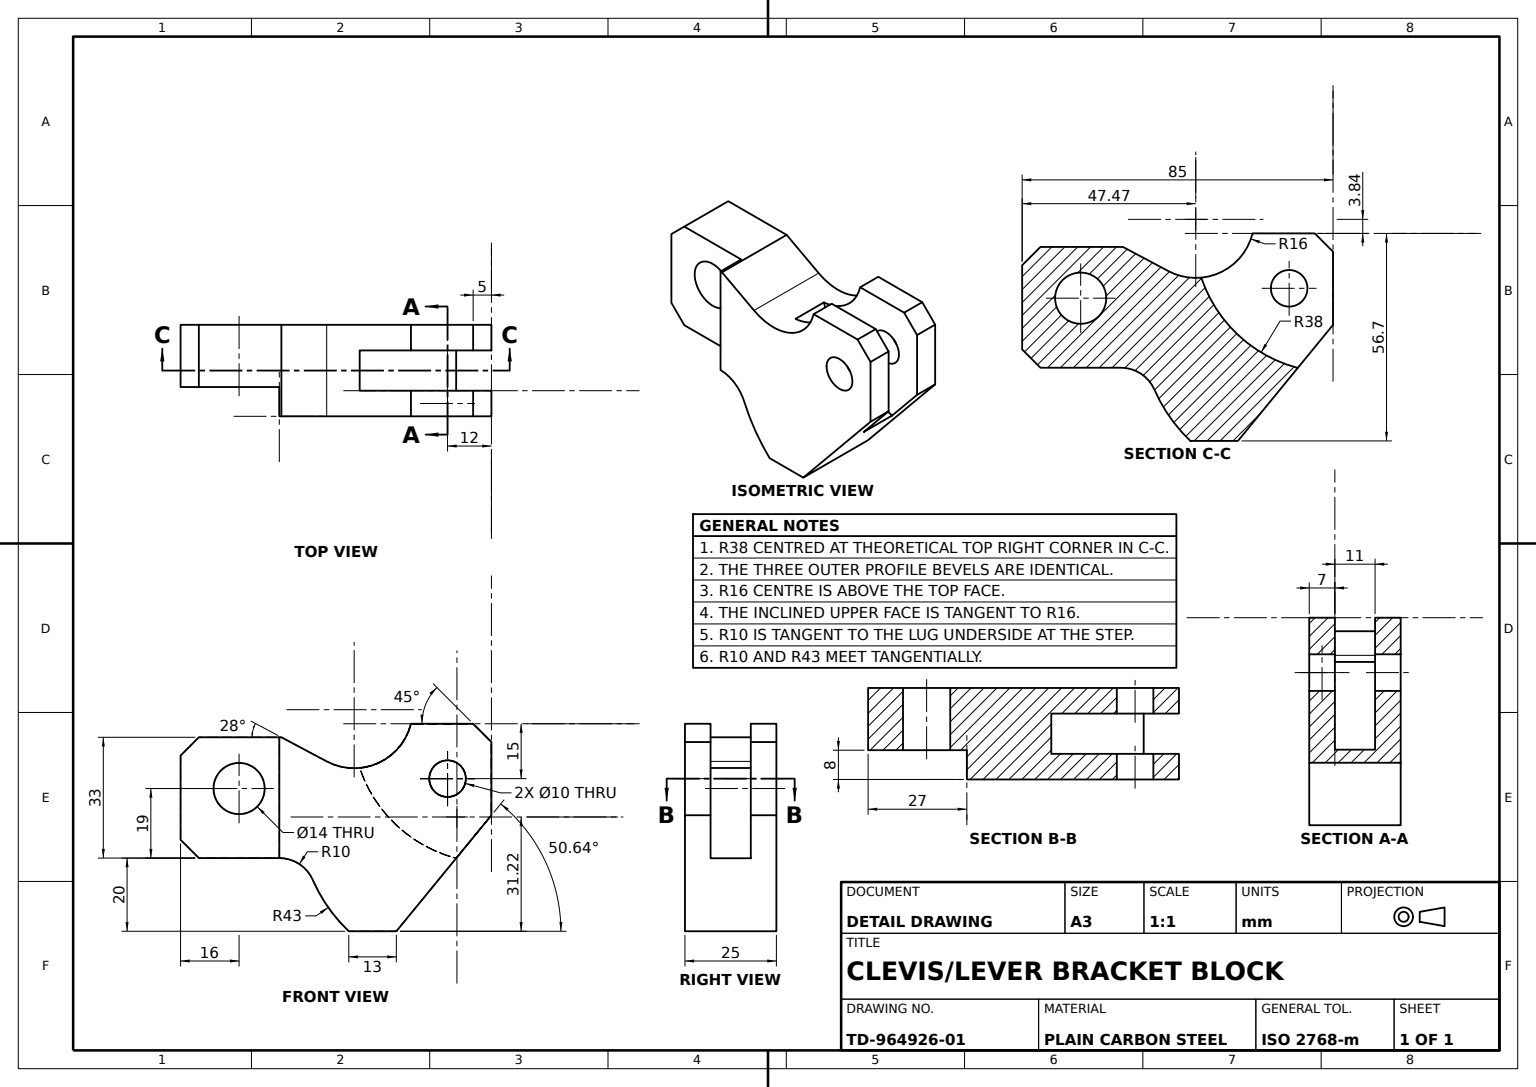
SolidWorks part; units mm, degrees
material "Plain Carbon Steel"
ref_plane "Front Plane" through (0, 0, 0) normal (0, 0, 1) x (1, 0, 0)
ref_plane "Top Plane" through (0, 0, 0) normal (0, 1, 0) x (1, 0, 0)
ref_plane "Right Plane" through (0, 0, 0) normal (1, 0, 0) x (0, 0, -1)
sketch "Bracket Profile Sketch" plane through (0, 0, 0) normal (0, 0, 1) x (1, 0, 0)
  line L0 (-1.4676, -60.5394) -> (11.5324, -60.5394)
  line L1 (32.5324, -3.84) -> (15.5324, -3.84)
  line L2 (37.5324, -8.84) -> (37.5324, -28.84)
  line L5 (11.5324, -60.5394) -> (37.5324, -28.84)
  line L6 (-19.9014, -7.5394) -> (-7.5115, -14.1272)
  line L7 (-47.4676, -12.5394) -> (-42.4676, -7.5394)
  line L8 (-42.4676, -7.5394) -> (-19.9014, -7.5394)
  line L9 (-47.4676, -12.5394) -> (-47.4676, -35.5394)
  line L10 (-42.4676, -40.5394) -> (-20.4679, -40.5394)
  line L12 (37.5324, -8.84) -> (32.5324, -3.84)
  line L13 (-47.4676, -35.5394) -> (-42.4676, -40.5394)
  circle A1 centre (25.5324, -18.84) radius 5
  arc A3 (-7.5115, -14.1272) -> (15.5324, -3.84) centre (0, 0) ccw
  circle A4 centre (-31.4676, -21.5394) radius 7
  arc A5 (-11.3047, -46.5348) -> (-20.4679, -40.5394) centre (-20.4679, -50.5394) ccw
  arc A8 (-1.4676, -60.5394) -> (-11.3047, -46.5348) centre (28.097, -29.3154) cw
  point P0 (37.5324, -3.84)
  point P5 (-47.4676, -7.5394)
  point P14 (-47.4676, -40.5394)
  point P16 (5.0324, -60.5394)
  dimension "D3" = 3.84
  dimension "D5" = 10
  dimension "D8" = 5
  dimension "D9" = 33
  dimension "D15" = 14
  dimension "D16" = 16
  dimension "D12" = 32
  dimension "D18" = 20
  dimension "D19" = 45
  dimension "D20" = 43
  dimension "D22" = 45
  dimension "D21" = 5
  dimension "D1" = 22
  dimension "D2" = 25
  dimension "D4" = 28
  dimension "D6" = 15
  dimension "D7" = 12
  dimension "D10" = 26
  dimension "D11" = 13
  dimension "D13" = 20
  dimension "D14" = 85
  dimension "D17" = 14
  dimension "D23" = 5
  dimension "D24" = 45
  dimension "D25" = 56.6994
  dimension "D26" = 21.9998
extrude "Bracket Body 25mm" add sketch "Bracket Profile Sketch" along normal mid plane 25
sketch "Fork Slot Sketch" plane through (0, 0, 0) normal (0, 1, 0) x (1, 0, 0)
  line L1 (-47.4676, -12.5) -> (-20.4676, -12.5)
  line L2 (-47.4676, -12.5) -> (-47.4676, -4.5)
  line L3 (-47.4676, -4.5) -> (-20.4676, -4.5)
  line L4 (-20.4676, -12.5) -> (-20.4676, -4.5)
  dimension "D1" = 27
  dimension "D2" = 8
extrude "Fork Slot 8x27" cut sketch "Fork Slot Sketch" against normal blind 63
sketch "Relief Circle Sketch Ø76" plane through (0, 0, 0) normal (0, 0, 1) x (1, 0, 0)
  circle A0 centre (37.5324, -3.84) radius 38
  dimension "D1" = 76
extrude "Front Relief Cut Ø76" cut sketch "Relief Circle Sketch Ø76" against normal mid plane 11
